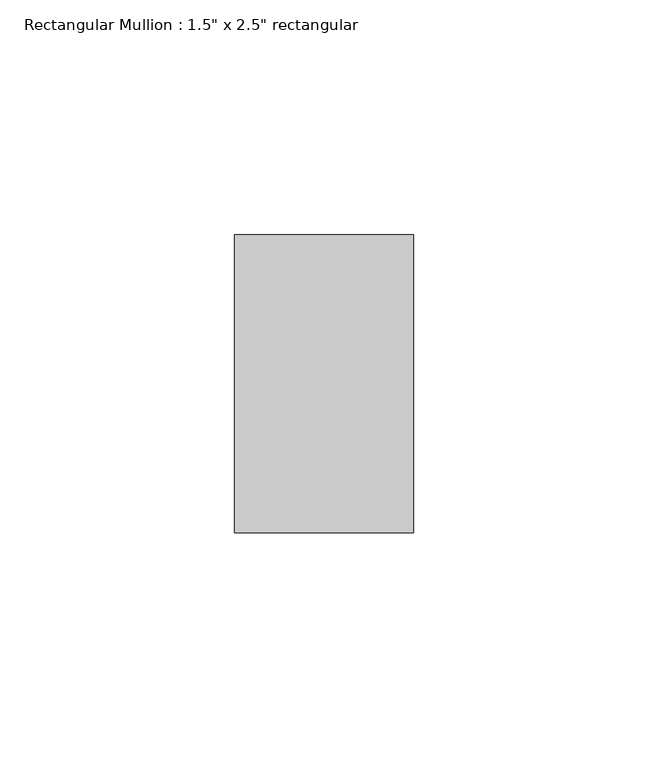
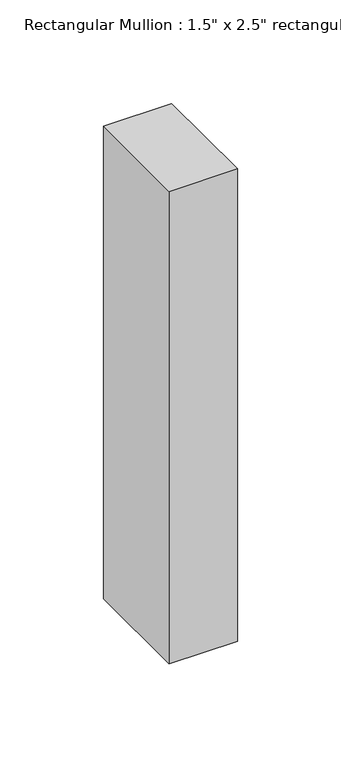
"""IFC4 building model written with IfcOpenShell, lengths in millimetres: member geometry."""

from ifc_helpers import new_model, si_unit, frame, origin, place, context, project, spatial, polyline, outline, extrude, source, transform, mapped, element, save


def member_01c630bb(model_context):
    return source(origin(), model_context, "Body", "SweptSolid", [
        extrude(outline(polyline([(19.05, 31.75), (19.05, -31.75), (-19.05, -31.75), (-19.05, 31.75), (19.05, 31.75)])), frame((0.0, 0.0, -278.5951523), z_axis=(0.0, 0.0, 1.0), x_axis=(1.0, 0.0, 0.0)), (0.0, 0.0, 1.0), 278.5951523),
    ])


if __name__ == "__main__":
    model = new_model("IFC4")
    model_context = context("Model", 3, world=origin())
    ifc_project = project(units=[si_unit("LENGTHUNIT", "METRE", prefix="MILLI")], contexts=[model_context])
    site = spatial("IfcSite", under=ifc_project)
    building = spatial("IfcBuilding", under=site)
    placement = place(None, origin())
    member_shape = member_01c630bb(model_context)
    element("IfcMember", 1, ObjectType="Rectangular Mullion : 1.5\" x 2.5\" rectangular", at=placement, inside=building, context=model_context, shape_type="MappedRepresentation", body=[
        mapped(member_shape, transform((0.0, 0.0, 0.0), x_axis=(1.0, 0.0, 0.0), y_axis=(0.0, 1.0, 0.0), z_axis=(0.0, 0.0, 1.0))),
    ])
    save(model, "model.ifc")

# Revit data of these elements
# Type "Rectangular Mullion : 1.5\" x 2.5\" rectangular"
#   built-in parameter 1007304 = 0.208333 (stored number, unit not read)
#   built-in parameter 1007301 = 0.0625 (stored number, unit not read)
#   built-in parameter 1007300 = 0.0625 (stored number, unit not read)
# Element 1 (IfcMember, "Rectangular Mullion : 1.5\" x 2.5\" rectangular")
#   Materials on its faces: "Leather - Black"
# Materials
#   "Leather - Black": class "Generic", colour RGB 40 40 40, transparency 0, Cost = 0
